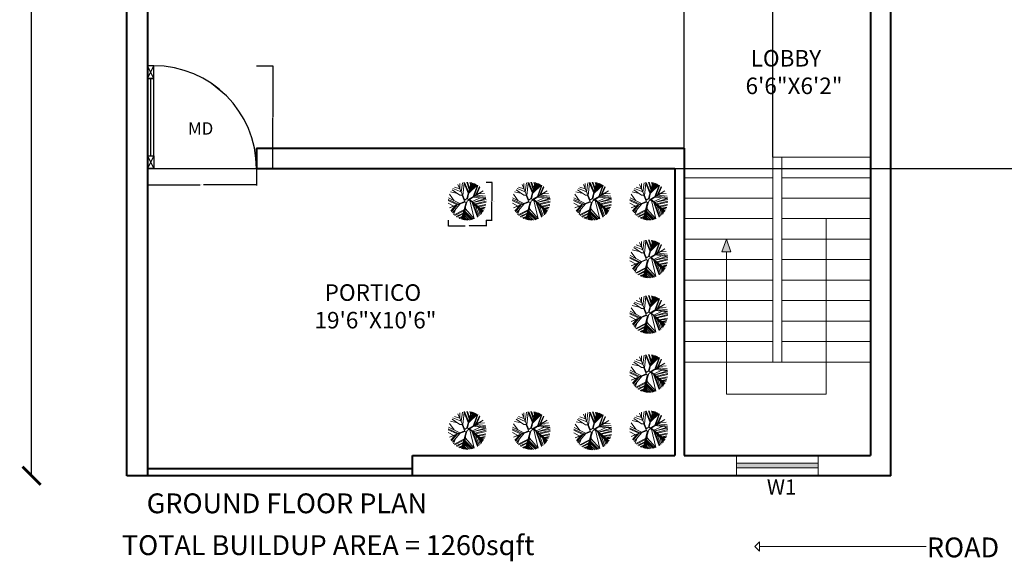
# Model space of a CAD drawing. Units: inches. Extents: x 182 to 1022, y -617 to 111.
# Tile 1 of 33: x 182 to 615, y -578 to -340. Entities that reach past the tile are written whole.
import ezdxf

# ---------------------------------------------------------------- set-up
doc = ezdxf.new("R2010")
doc.units = ezdxf.units.IN
doc.header["$MEASUREMENT"] = 0
for name, color, linetype, lineweight in [('A-ANNO-DIMS', 2, 'Continuous', 18), ('A-ANNO-IDEN', 1, 'Continuous', 18), ('A-ANNO-PATT', 1, 'Continuous', 15), ('A-ANNO-SYMB', 1, 'Continuous', 15), ('A-ANNO-TEXT', 8, 'Continuous', 20), ('A-AREA-IDEN', 8, 'Continuous', 18), ('A-FLOR-STRS', 1, 'Continuous', 20), ('A-GLAZ-PATT', 5, 'Continuous', 13), ('door', 2, 'Continuous', 25), ('wall', 1, 'Continuous', 40), ('wind', 5, 'Continuous', 20)]:
    doc.layers.add(name, color=color, linetype=linetype, lineweight=lineweight)
doc.layers.add('GRASS', color=90, linetype='Continuous', lineweight=13, transparency=0.7)
doc.styles.get("Standard").update_dxf_attribs({"font": 'arial.ttf'})
doc.dimstyles.get("Standard").update_dxf_attribs({"dimtxt": 0.18, "dimasz": 0.18, "dimexe": 0.18, "dimexo": 0.0625, "dimgap": 0.09, "dimtad": 0, "dimtih": 1, "dimtoh": 1, "dimdec": 1, "dimzin": 0, "dimdsep": 46, "dimlunit": 4, "dimtxsty": 'Standard', "dimcen": 0.09, "dimadec": 0, "dimazin": 0, "dimtfac": 1, "dimtdec": 1, "dimtofl": 0, "dimtmove": 0, "dimatfit": 3, "dimfxl": 1, "dimtolj": 1, "dimtzin": 0, "dimarcsym": 0})

# ---------------------------------------------------------------- blocks, each defined once
blk = doc.blocks.new('A$C2D7661C6')
for p, q in [((0, 700), (50, 800)), ((50, 700), (0, 800)), ((25, 700), (25, 100)), ((50, 100), (0, 0)), ((0, 100), (50, 0))]:
    blk.add_line(p, q)
for points in [[(0, 700), (50, 700), (50, 800), (0, 800)], [(0, 100), (50, 100), (50, 700), (0, 700)], [(0, 100), (50, 100), (50, 0), (0, 0)]]:
    blk.add_lwpolyline(points, close=True)
blk.add_arc((50, 0), 800, 0, 90)
blk = doc.blocks.new('A$C7F556C88')
for p, q in [((615.7, 565.7), (500.3, 661.3)), ((50, 0), (850, 0))]:
    blk.add_line(p, q)
blk.add_blockref('A$C2D7661C6', (0, 0))
blk = doc.blocks.new('A$C4FA53466')
at = {"color": 0}
for p, q in [((0.506, 1.079), (0.165, 1.314)), ((0.562, 1.217), (0.205, 1.363)), ((0.505, 1.347), (0.266, 1.426)), ((0.717, 0.864), (0.422, 1.538)), ((0.501, 1.356), (0.505, 1.578)), ((0.563, 1.216), (0.612, 1.614)), ((0.627, 1.07), (0.687, 1.601)), ((0.867, 1.166), (0.675, 1.628)), ((0.882, 1.223), (0.709, 1.633)), ((0.91, 1.328), (0.802, 1.64)), ((0.988, 1.623), (0.804, 0.931)), ((0.925, 1.384), (0.834, 1.64)), ((0.836, 0.927), (0.988, 1.623)), ((0.887, 1.159), (1.256, 1.515)), ((0.901, 1.223), (1.228, 1.532)), ((0.914, 1.283), (1.197, 1.549)), ((0.922, 1.323), (1.176, 1.559)), ((0.964, 1.534), (0.938, 1.632)), ((0.938, 1.393), (1.132, 1.579)), ((0.945, 1.425), (1.104, 1.59)), ((0.967, 1.545), (0.952, 1.63)), ((0.965, 1.517), (1.059, 1.605)), ((0.974, 1.559), (1.002, 1.62)), ((1.085, 1.015), (1.262, 1.512)), ((1.121, 1.036), (1.274, 1.503)), ((1.18, 1.071), (1.349, 1.447)), ((1.222, 1.096), (1.37, 1.428)), ((0.436, 0.689), (0.003, 0.892)), ((0.501, 0.716), (0.012, 0.965)), ((0.255, 0.841), (0.055, 1.116)), ((0.406, 1.148), (0.102, 1.217)), ((0.614, 1.092), (0.506, 1.079)), ((0.604, 1.069), (0.506, 1.079)), ((0.715, 0.784), (0.604, 1.069)), ((0.804, 0.931), (0.717, 0.864)), ((0.82, 0.82), (0.904, 0.875)), ((0.879, 0.894), (0.836, 0.927)), ((1.509, 1.265), (0.879, 0.894)), ((1.521, 0.394), (0.904, 0.875)), ((0.926, 0.889), (1.509, 1.265)), ((0.926, 0.889), (1.521, 0.394)), ((1.03, 0.802), (1.392, 0.963)), ((1.073, 0.767), (1.614, 0.936)), ((1.081, 0.769), (1.638, 0.886)), ((1.097, 0.999), (1.632, 0.934)), ((1.148, 1.032), (1.626, 0.972)), ((1.211, 1.073), (1.612, 1.034)), ((1.3, 1.13), (1.573, 1.147)), ((0.384, 0.667), (0, 0.848)), ((0.237, 0.605), (0.004, 0.735)), ((0.053, 0.528), (0.708, 0.803)), ((0.716, 0.781), (0.053, 0.528)), ((0.321, 0.63), (0.115, 0.4)), ((0.387, 0.655), (0.137, 0.366)), ((0.516, 0.704), (0.179, 0.309)), ((0.313, 0.466), (0.232, 0.248)), ((0.682, 0.44), (0.255, 0.225)), ((0.82, 0.82), (0.575, 0.037)), ((0.575, 0.037), (0.769, 0.772)), ((0.701, 0.44), (0.621, 0.024)), ((0.732, 0.539), (0.664, 0.015)), ((0.737, 0.554), (0.691, 0.01)), ((0.715, 0.784), (0.775, 0.767)), ((0.744, 0.569), (0.717, 0.006)), ((0.74, 0.488), (1.121, 0.057)), ((0.938, 0.848), (1.126, 0.059)), ((1.016, 0.788), (1.263, 0.13)), ((1.04, 0.769), (1.475, 0.326)), ((1.06, 0.754), (1.5, 0.362)), ((1.083, 0.725), (1.298, 0.153)), ((1.153, 0.701), (1.64, 0.826)), ((1.161, 0.646), (1.335, 0.182)), ((1.185, 0.674), (1.639, 0.776)), ((1.273, 0.601), (1.627, 0.672)), ((1.298, 0.58), (1.618, 0.629)), ((1.301, 0.503), (1.386, 0.227)), ((1.365, 0.438), (1.42, 0.26)), ((1.376, 0.515), (1.599, 0.562)), ((1.392, 0.502), (1.593, 0.545)), ((1.412, 0.486), (1.569, 0.486)), ((0.673, 0.407), (0.281, 0.201)), ((0.645, 0.301), (0.342, 0.153)), ((0.636, 0.267), (0.375, 0.133)), ((0.608, 0.161), (0.439, 0.093)), ((0.6, 0.133), (0.475, 0.076)), ((0.59, 0.094), (0.501, 0.064)), ((0.72, 0.07), (0.793, 0)), ((0.722, 0.111), (0.842, 0)), ((0.726, 0.192), (0.924, 0.006)), ((0.73, 0.277), (0.998, 0.019)), ((0.733, 0.326), (1.037, 0.029)), ((0.735, 0.369), (1.067, 0.038)), ((1.413, 0.39), (1.444, 0.288))]:
    blk.add_line(p, q, dxfattribs=at)
blk = doc.blocks.new('_ArchTick')
at = {"color": 0, "linetype": 'ByBlock', "const_width": 0.15}
blk.add_lwpolyline([(-0.5, -0.5), (0.5, 0.5)], dxfattribs=at)
blk = doc.blocks.new('*D6')
at = {"layer": 'A-ANNO-DIMS', "color": 0, "lineweight": -2, "transparency": 16777216}
for p, q in [((187.47, -0.37), (187.47, -260.42)), ((187.47, -540.37), (187.47, -280.32))]:
    blk.add_line(p, q, dxfattribs=at)
at = {"layer": 'Defpoints', "color": 0, "transparency": 16777216}
for p in [(229.36, -0.37), (187.47, -540.37), (229.36, -540.37)]:
    blk.add_point(p, dxfattribs=at)
at = {"layer": 'A-ANNO-DIMS', "color": 0, "lineweight": -2, "transparency": 16777216, "xscale": 8, "yscale": 8, "zscale": 8}
for p, rotation in [((187.47, -0.37), 90), ((187.47, -540.37), 270)]:
    blk.add_blockref('_ArchTick', p, dxfattribs=dict(at, rotation=rotation))
at = {"layer": 'A-ANNO-DIMS', "color": 0, "transparency": 16777216, "insert": (187.47, -270.37), "char_height": 8, "attachment_point": 5, "rotation": 90}
blk.add_mtext("\\A1;45'", dxfattribs=at)
blk = doc.blocks.new('STAIR-DOGLEG')
for p, q in [((39, 0), (39, 90)), ((39, 90), (82, 90)), ((43, 0), (43, 90)), ((0, 81), (39, 81)), ((43, 81), (82, 81)), ((0, 72), (39, 72)), ((43, 72), (82, 72)), ((0, 63), (39, 63)), ((43, 63), (82, 63)), ((0, 54), (39, 54)), ((43, 54), (82, 54)), ((0, 45), (39, 45)), ((43, 45), (82, 45)), ((0, 36), (39, 36)), ((43, 36), (82, 36)), ((0, 27), (39, 27)), ((43, 27), (82, 27)), ((0, 18), (39, 18)), ((43, 18), (82, 18)), ((0, 9), (39, 9)), ((43, 9), (82, 9)), ((0, 0), (82, 0))]:
    blk.add_line(p, q)
blk = doc.blocks.new('*D18')
at = {"layer": 'A-ANNO-DIMS', "color": 0, "lineweight": -2, "transparency": 16777216}
for p, q in [((238.36, -405.44), (238.36, -412.75)), ((286.36, -405.44), (286.36, -412.75)), ((238.54, -412.57), (261.63, -412.57)), ((286.18, -412.57), (263.1, -412.57))]:
    blk.add_line(p, q, dxfattribs=at)
at = {"layer": 'A-ANNO-DIMS', "color": 0, "transparency": 16777216}
for points in [[(238.54, -412.54), (238.54, -412.6), (238.36, -412.57)], [(286.18, -412.54), (286.18, -412.6), (286.36, -412.57)]]:
    blk.add_solid(points, dxfattribs=at)
at = {"layer": 'Defpoints', "color": 0, "transparency": 16777216}
for p in [(238.36, -405.37), (286.36, -405.37), (286.36, -412.57)]:
    blk.add_point(p, dxfattribs=at)
at = {"layer": 'A-ANNO-DIMS', "color": 0, "transparency": 16777216, "insert": (262.36, -412.57), "char_height": 0.18, "attachment_point": 5}
blk.add_mtext('\\A1;DOOR 4\'-0"', dxfattribs=at)
blk = doc.blocks.new('*D19')
at = {"layer": 'A-ANNO-DIMS', "color": 0, "lineweight": -2, "transparency": 16777216}
for p, q in [((286.42, -360.2), (293.74, -360.2)), ((293.56, -360.38), (293.56, -382.6)), ((293.56, -405.19), (293.56, -382.97)), ((286.42, -405.37), (293.74, -405.37))]:
    blk.add_line(p, q, dxfattribs=at)
at = {"layer": 'A-ANNO-DIMS', "color": 0, "transparency": 16777216}
for points in [[(293.53, -360.38), (293.59, -360.38), (293.56, -360.2)], [(293.53, -405.19), (293.59, -405.19), (293.56, -405.37)]]:
    blk.add_solid(points, dxfattribs=at)
at = {"layer": 'Defpoints', "color": 0, "transparency": 16777216}
for p in [(286.36, -360.2), (293.56, -360.2), (286.36, -405.37)]:
    blk.add_point(p, dxfattribs=at)
at = {"layer": 'A-ANNO-DIMS', "color": 0, "transparency": 16777216, "insert": (293.56, -382.79), "char_height": 0.18, "attachment_point": 5}
blk.add_mtext('\\A1;3\'-9"', dxfattribs=at)
blk = doc.blocks.new('*D30')
at = {"layer": 'A-ANNO-DIMS', "color": 0, "lineweight": -2, "transparency": 16777216}
for p, q in [((387.41, -411.35), (390.03, -411.35)), ((389.85, -411.53), (389.85, -419.51)), ((389.85, -427.85), (389.85, -419.88)), ((387.41, -428.03), (390.03, -428.03))]:
    blk.add_line(p, q, dxfattribs=at)
at = {"layer": 'A-ANNO-DIMS', "color": 0, "transparency": 16777216}
for points in [[(389.82, -411.53), (389.88, -411.53), (389.85, -411.35)], [(389.82, -427.85), (389.88, -427.85), (389.85, -428.03)]]:
    blk.add_solid(points, dxfattribs=at)
at = {"layer": 'Defpoints', "color": 0, "transparency": 16777216}
for p in [(387.34, -411.35), (389.85, -411.35), (387.34, -428.03)]:
    blk.add_point(p, dxfattribs=at)
at = {"layer": 'A-ANNO-DIMS', "color": 0, "transparency": 16777216, "insert": (389.85, -419.69), "char_height": 0.18, "attachment_point": 5}
blk.add_mtext('\\A1;PLANT 1\'-4 1/2" TYP.', dxfattribs=at)
blk = doc.blocks.new('*D31')
at = {"layer": 'A-ANNO-DIMS', "color": 0, "lineweight": -2, "transparency": 16777216}
for p, q in [((370.66, -428.1), (370.66, -430.72)), ((387.34, -428.1), (387.34, -430.72)), ((370.84, -430.54), (378.16, -430.54)), ((387.16, -430.54), (379.84, -430.54))]:
    blk.add_line(p, q, dxfattribs=at)
at = {"layer": 'A-ANNO-DIMS', "color": 0, "transparency": 16777216}
for points in [[(370.84, -430.51), (370.84, -430.57), (370.66, -430.54)], [(387.16, -430.51), (387.16, -430.57), (387.34, -430.54)]]:
    blk.add_solid(points, dxfattribs=at)
at = {"layer": 'Defpoints', "color": 0, "transparency": 16777216}
for p in [(370.66, -428.03), (387.34, -428.03), (387.34, -430.54)]:
    blk.add_point(p, dxfattribs=at)
at = {"layer": 'A-ANNO-DIMS', "color": 0, "transparency": 16777216, "insert": (379, -430.54), "char_height": 0.18, "attachment_point": 5}
blk.add_mtext('\\A1;1\'-4 1/2" TYP.', dxfattribs=at)
blk = doc.blocks.new('*D39')
at = {"layer": 'A-ANNO-DIMS', "color": 0, "lineweight": -2, "transparency": 16777216}
for p, q in [((238.4, -288.54), (1015.28, -288.54)), ((1015.1, -288.72), (1015.1, -346.77)), ((1015.1, -405.19), (1015.1, -347.14)), ((238.43, -405.37), (1015.28, -405.37))]:
    blk.add_line(p, q, dxfattribs=at)
at = {"layer": 'A-ANNO-DIMS', "color": 0, "transparency": 16777216}
for points in [[(1015.07, -288.72), (1015.13, -288.72), (1015.1, -288.54)], [(1015.07, -405.19), (1015.13, -405.19), (1015.1, -405.37)]]:
    blk.add_solid(points, dxfattribs=at)
at = {"layer": 'Defpoints', "color": 0, "transparency": 16777216}
for p in [(238.34, -288.54), (1015.1, -288.54), (238.36, -405.37)]:
    blk.add_point(p, dxfattribs=at)
at = {"layer": 'A-ANNO-DIMS', "color": 0, "transparency": 16777216, "insert": (1015.1, -346.96), "char_height": 0.18, "attachment_point": 5}
blk.add_mtext('\\A1;9\'-9"', dxfattribs=at)
blk = doc.blocks.new('*D47')
at = {"layer": 'A-ANNO-DIMS', "color": 0, "lineweight": -2, "transparency": 16777216}
for p, q in [((474.36, -396.31), (474.36, 42.61)), ((474.54, 42.43), (493.53, 42.43)), ((513.18, 42.43), (494.19, 42.43)), ((513.36, -400.31), (513.36, 42.61))]:
    blk.add_line(p, q, dxfattribs=at)
at = {"layer": 'A-ANNO-DIMS', "color": 0, "transparency": 16777216}
for points in [[(474.54, 42.46), (474.54, 42.4), (474.36, 42.43)], [(513.18, 42.46), (513.18, 42.4), (513.36, 42.43)]]:
    blk.add_solid(points, dxfattribs=at)
at = {"layer": 'Defpoints', "color": 0, "transparency": 16777216}
for p in [(513.36, 42.43), (474.36, -396.37), (513.36, -400.37)]:
    blk.add_point(p, dxfattribs=at)
at = {"layer": 'A-ANNO-DIMS', "color": 0, "transparency": 16777216, "insert": (493.86, 42.43), "char_height": 0.18, "attachment_point": 5}
blk.add_mtext('\\A1;3\'-3"', dxfattribs=at)

msp = doc.modelspace()

# ---------------------------------------------------------------- hatches: boundary and pattern name
at = {"layer": 'A-ANNO-PATT'}
h = msp.add_hatch(color=256, dxfattribs=at)
h.dxf.hatch_style = 1
h.paths.add_polyline_path([(492.96, -436.37), (490.96, -442.01), (492.96, -442.01), (494.96, -442.01)])
h.paths.add_polyline_path([(899.9, -436.37), (897.9, -442.01), (899.9, -442.01), (901.9, -442.01)])
at = {"layer": 'A-GLAZ-PATT'}
h = msp.add_hatch(color=256, dxfattribs=at)
h.dxf.hatch_style = 1
h.paths.add_polyline_path([(285.4, -3.87), (255.4, -3.87), (255.4, -5.87), (285.4, -5.87)])
h.paths.add_polyline_path([(376.09, -3.87), (340.09, -3.87), (340.09, -5.87), (376.09, -5.87)])
h.paths.add_polyline_path([(561.86, -132.92), (559.86, -132.92), (559.86, -168.92), (561.86, -168.92)])
h.paths.add_polyline_path([(561.86, -56.81), (559.86, -56.81), (559.86, -86.81), (561.86, -86.81)])
h.paths.add_polyline_path([(561.86, -258.37), (559.86, -258.37), (559.86, -282.37), (561.86, -282.37)])
h.paths.add_polyline_path([(533.36, -534.87), (497.36, -534.87), (497.36, -536.87), (533.36, -536.87)])
h.paths.add_polyline_path([(234.86, -252.37), (232.86, -252.37), (232.86, -288.37), (234.86, -288.37)])

# ---------------------------------------------------------------- linework, layer by layer
at = {"layer": 'A-ANNO-SYMB'}
for p, q in [((536.86, -427.37), (536.86, -504.45)), ((492.96, -436.37), (490.96, -442.01)), ((492.96, -436.37), (494.96, -442.01)), ((492.96, -442.01), (490.96, -442.01)), ((492.96, -504.45), (492.96, -442.01)), ((492.96, -442.01), (494.96, -442.01)), ((536.86, -504.45), (492.96, -504.45)), ((505.47, -571.43), (507.47, -569.43)), ((505.47, -571.43), (507.47, -573.43)), ((507.47, -571.43), (507.47, -569.43)), ((580.87, -571.43), (507.47, -571.43)), ((507.47, -571.43), (507.47, -573.43))]:
    msp.add_line(p, q, dxfattribs=at)
at = {"layer": 'wall'}
for p, q in [((229.36, -540.37), (229.36, -0.37)), ((565.36, -540.37), (565.36, -0.37)), ((238.36, -9.37), (238.36, -540.37)), ((556.36, -246.37), (556.36, -531.37)), ((286.36, -396.37), (474.36, -396.37)), ((286.36, -396.37), (286.36, -405.37)), ((474.36, -396.37), (474.36, -531.37)), ((286.36, -405.37), (470.36, -405.37)), ((470.36, -405.37), (470.36, -531.37)), ((354.94, -531.37), (470.36, -531.37)), ((354.94, -540.37), (354.94, -531.37)), ((474.36, -531.37), (556.36, -531.37)), ((565.36, -540.37), (229.36, -540.37)), ((354.94, -537.37), (238.36, -537.37))]:
    msp.add_line(p, q, dxfattribs=at)
at = {"layer": 'wind'}
for p, q in [((497.36, -531.37), (497.36, -540.37)), ((533.36, -531.37), (533.36, -540.37)), ((497.36, -534.87), (533.36, -534.87)), ((497.36, -536.87), (533.36, -536.87))]:
    msp.add_line(p, q, dxfattribs=at)

# ---------------------------------------------------------------- block references
at = {"layer": 'A-FLOR-STRS'}
msp.add_blockref('STAIR-DOGLEG', (474.36, -490.37), dxfattribs=at)
at = {"layer": 'door', "xscale": 0.0564669652975506, "yscale": 0.0564669652975506, "zscale": 0.0564669652975506}
msp.add_blockref('A$C7F556C88', (238.36, -405.37), dxfattribs=at)
at = {"layer": 'GRASS', "xscale": 10.16810711056296, "yscale": 10.16810711056296, "zscale": 10.16810711056296}
for p in [(370.66, -428.03), (398.83, -428.03), (425.81, -428.03), (450.54, -428.03), (450.54, -453.43), (450.54, -477.87), (450.54, -503.76), (370.66, -528.77), (398.83, -528.81), (425.9, -528.98), (450.54, -528.48)]:
    msp.add_blockref('A$C4FA53466', p, dxfattribs=at)

# ---------------------------------------------------------------- texts
at = {"layer": 'A-ANNO-IDEN'}
for s, height, p in [('MD', 5.444, (256.22, -390.46)), ('W1', 6.652, (510.78, -548.62))]:
    msp.add_text(s, height=height, dxfattribs=at).set_placement(p)
at = {"layer": 'A-ANNO-TEXT', "attachment_point": 1}
for s, width, insert, char_height in [(' GROUND FLOOR PLAN', 146.1965, (235.4, -548.1), 8.7185), ('TOTAL BUILDUP AREA = 1260sqft', 195.6714, (227.18, -566.48), 8.7185), (' ROAD', 39.5481, (578.47, -567.47), 8.718)]:
    msp.add_mtext_dynamic_manual_height_columns(s, width=width, gutter_width=1.45, heights=[0], dxfattribs=dict(at, insert=insert, char_height=char_height))
at = {"layer": 'A-AREA-IDEN', "char_height": 7.2703, "attachment_point": 1}
for s, width, insert in [(' LOBBY      6\'6"X6\'2"', 42.598, (501.41, -353.27)), ('  PORTICO\\P 19\'6"X10\'6"', 54.6851, (311.85, -456.22))]:
    msp.add_mtext_dynamic_manual_height_columns(s, width=width, gutter_width=1.21, heights=[0], dxfattribs=dict(at, insert=insert))

# ---------------------------------------------------------------- dimensions: what is measured, and where the dimension line sits
at = {"layer": 'A-ANNO-DIMS'}
dim = msp.add_linear_dim(base=(513.36, 42.43), p1=(474.36, -396.37), p2=(513.36, -400.37), dimstyle='Standard', override={"dimdec": 1, "dimlfac": 1, "dimrnd": 0, "dimzin": 1, "dimdsep": 46, "dimlunit": 4, "dimfrac": 2}, dxfattribs=at)
dim.commit()
dim.dimension.update_dxf_attribs({"geometry": '*D47', "text_midpoint": (493.86, 42.43)})
for base, p1, p2, override, picture, middle in [((187.47, -540.37), (229.36, -0.37), (229.36, -540.37), {"dimtxt": 8, "dimasz": 8, "dimgap": 3, "dimtih": 0, "dimblk1": 'ArchTick', "dimblk2": 'ArchTick', "dimsah": 1, "dimse1": 1, "dimse2": 1, "dimclrd": 0, "dimclre": 0, "dimclrt": 0}, '*D6', (187.47, -270.37)), ((1015.1, -288.54), (238.36, -405.37), (238.34, -288.54), {"dimdec": 1, "dimlfac": 1, "dimrnd": 0, "dimzin": 1, "dimdsep": 46, "dimlunit": 4, "dimfrac": 2}, '*D39', (1015.1, -346.96)), ((293.56, -360.2), (286.36, -405.37), (286.36, -360.2), {"dimdec": 1, "dimlfac": 1, "dimrnd": 0, "dimzin": 1, "dimdsep": 46, "dimlunit": 4, "dimfrac": 2}, '*D19', (293.56, -382.79))]:
    dim = msp.add_linear_dim(base=base, p1=p1, p2=p2, angle=90, dimstyle='Standard', override=override, dxfattribs=at)
    dim.commit()
    dim.dimension.update_dxf_attribs({"geometry": picture, "text_midpoint": middle})
for base, p1, p2, text, picture, middle in [((286.36, -412.57), (238.36, -405.37), (286.36, -405.37), 'DOOR <>', '*D18', (262.36, -412.57)), ((387.34, -430.54), (370.66, -428.03), (387.34, -428.03), '<> TYP.', '*D31', (379, -430.54))]:
    dim = msp.add_linear_dim(base=base, p1=p1, p2=p2, text=text, dimstyle='Standard', override={"dimdec": 1, "dimlfac": 1, "dimrnd": 0, "dimzin": 1, "dimdsep": 46, "dimlunit": 4, "dimfrac": 2}, dxfattribs=at)
    dim.commit()
    dim.dimension.update_dxf_attribs({"geometry": picture, "text_midpoint": middle})
dim = msp.add_linear_dim(base=(389.85, -411.35), p1=(387.34, -428.03), p2=(387.34, -411.35), angle=90, text='PLANT <> TYP.', dimstyle='Standard', override={"dimdec": 1, "dimlfac": 1, "dimrnd": 0, "dimzin": 1, "dimdsep": 46, "dimlunit": 4, "dimfrac": 2}, dxfattribs=at)
dim.commit()
dim.dimension.update_dxf_attribs({"geometry": '*D30', "text_midpoint": (389.85, -419.69)})

doc.saveas('drawing.dxf')
